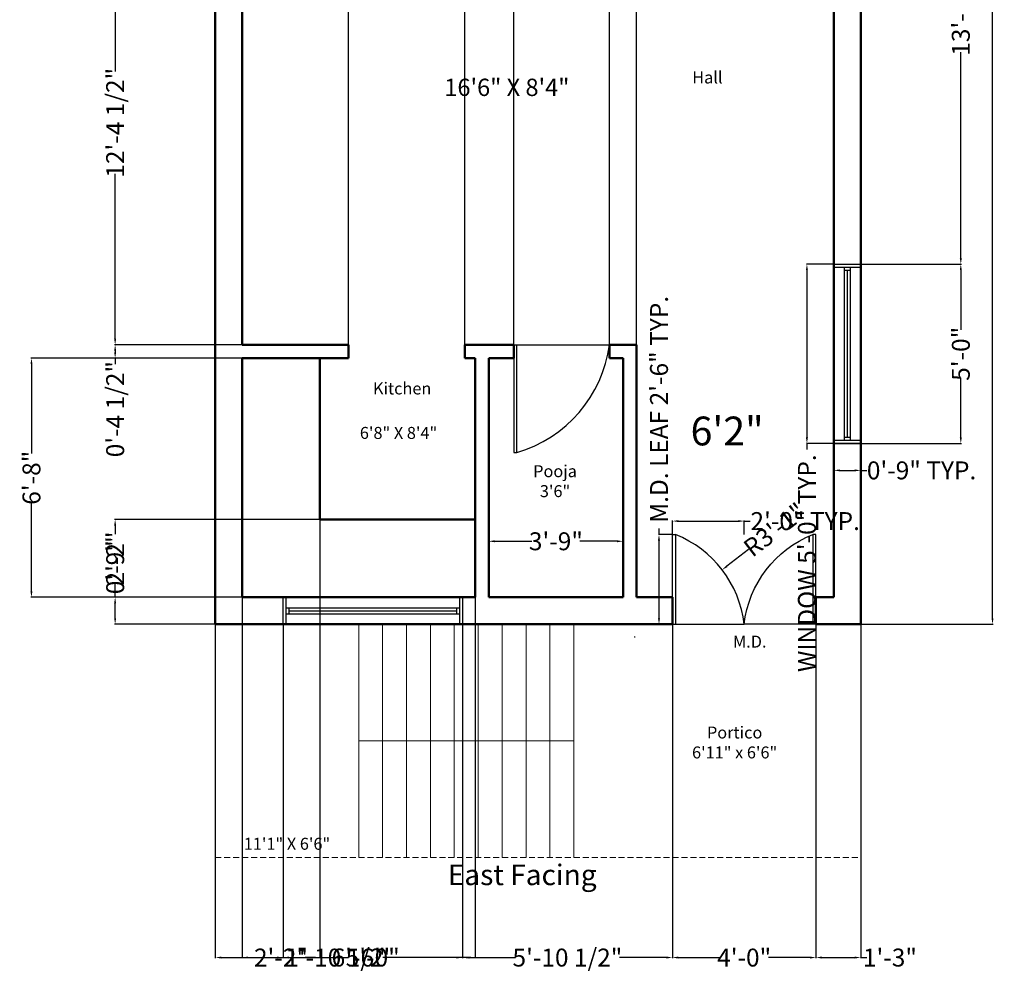
# Model space of a CAD drawing. Units: inches. Extents: x -34 to 296, y -84 to 618.
# Tile 1 of 3: x -34 to 296, y -84 to 238. Entities that reach past the tile are written whole.
import ezdxf

# ---------------------------------------------------------------- set-up
doc = ezdxf.new("R2010")
doc.units = ezdxf.units.IN
doc.header["$LTSCALE"] = 4
doc.header["$MEASUREMENT"] = 0
doc.linetypes.add('DASHED', pattern=[0.75, 0.5, -0.25])
for name, color, linetype, lineweight in [('A-ANNO-DIMS', 2, 'Continuous', 18), ('A-ANNO-TEXT', 7, 'Continuous', 18), ('A-AREA-IDEN', 3, 'Continuous', 18), ('A-DOOR', 4, 'Continuous', 25), ('A-FLOR-OVHD', 8, 'DASHED', 18), ('A-FLOR-STRS', 8, 'Continuous', 18), ('A-GLAZ', 3, 'Continuous', 25), ('A-WALL', 7, 'Continuous', 50)]:
    doc.layers.add(name, color=color, linetype=linetype, lineweight=lineweight)
doc.styles.get("Standard").update_dxf_attribs({"font": 'arial.ttf'})
doc.dimstyles.get("Standard").update_dxf_attribs({"dimtxt": 6, "dimasz": 2, "dimexe": 0.18, "dimexo": 0.0625, "dimgap": 0.09, "dimtad": 0, "dimdec": 0, "dimzin": 0, "dimdsep": 46, "dimlunit": 4, "dimtxsty": 'Standard', "dimcen": 0.09, "dimadec": 0, "dimazin": 0, "dimtfac": 1, "dimtdec": 0, "dimtofl": 0, "dimtmove": 0, "dimatfit": 3, "dimfxl": 1, "dimtolj": 1, "dimtzin": 0, "dimarcsym": 0})

# ---------------------------------------------------------------- blocks, each defined once
blk = doc.blocks.new('*D2')
at = {"layer": 'A-ANNO-DIMS', "color": 0, "lineweight": -2, "transparency": 16777216}
for p, q in [((247.53, 576.03), (291.77, 576.03)), ((291.59, 574.03), (291.59, 311.33)), ((291.59, 38.03), (291.59, 300.73)), ((247.53, 36.03), (291.77, 36.03))]:
    blk.add_line(p, q, dxfattribs=at)
at = {"layer": 'A-ANNO-DIMS', "color": 0, "transparency": 16777216}
for points in [[(291.26, 574.03), (291.92, 574.03), (291.59, 576.03)], [(291.26, 38.03), (291.92, 38.03), (291.59, 36.03)]]:
    blk.add_solid(points, dxfattribs=at)
at = {"layer": 'Defpoints', "color": 0, "transparency": 16777216}
for p in [(247.47, 576.03), (247.47, 36.03), (291.59, 36.03)]:
    blk.add_point(p, dxfattribs=at)
at = {"layer": 'A-ANNO-DIMS', "color": 0, "transparency": 16777216, "insert": (291.59, 306.03), "char_height": 6, "attachment_point": 5, "rotation": 90}
blk.add_mtext("\\A1;45'", dxfattribs=at)
blk = doc.blocks.new('*D3')
at = {"layer": 'A-ANNO-DIMS', "color": 0, "lineweight": -2, "transparency": 16777216}
for p, q in [((40.4, 125.03), (-30.22, 125.03)), ((-30.04, 123.03), (-30.04, 93.11)), ((-30.04, 47.03), (-30.04, 76.95)), ((40.4, 45.03), (-30.22, 45.03))]:
    blk.add_line(p, q, dxfattribs=at)
at = {"layer": 'A-ANNO-DIMS', "color": 0, "transparency": 16777216}
for points in [[(-30.37, 123.03), (-29.7, 123.03), (-30.04, 125.03)], [(-30.37, 47.03), (-29.7, 47.03), (-30.04, 45.03)]]:
    blk.add_solid(points, dxfattribs=at)
at = {"layer": 'Defpoints', "color": 0, "transparency": 16777216}
for p in [(-30.04, 125.03), (40.47, 125.03), (40.47, 45.03)]:
    blk.add_point(p, dxfattribs=at)
at = {"layer": 'A-ANNO-DIMS', "color": 0, "transparency": 16777216, "insert": (-30.04, 85.03), "char_height": 6, "attachment_point": 5, "rotation": 90}
blk.add_mtext('\\A1;6\'-8"', dxfattribs=at)
blk = doc.blocks.new('*D4')
at = {"layer": 'A-ANNO-DIMS', "color": 0, "lineweight": -2, "transparency": 16777216}
for p, q in [((122.97, 45.1), (122.97, 63.96)), ((124.97, 63.78), (137.4, 63.78)), ((165.97, 63.78), (153.53, 63.78)), ((167.97, 45.1), (167.97, 63.96))]:
    blk.add_line(p, q, dxfattribs=at)
at = {"layer": 'A-ANNO-DIMS', "color": 0, "transparency": 16777216}
for points in [[(124.97, 64.11), (124.97, 63.45), (122.97, 63.78)], [(165.97, 64.11), (165.97, 63.45), (167.97, 63.78)]]:
    blk.add_solid(points, dxfattribs=at)
at = {"layer": 'Defpoints', "color": 0, "transparency": 16777216}
for p in [(122.97, 63.78), (122.97, 45.03), (167.97, 45.03)]:
    blk.add_point(p, dxfattribs=at)
at = {"layer": 'A-ANNO-DIMS', "color": 0, "transparency": 16777216, "insert": (145.47, 63.78), "char_height": 6, "attachment_point": 5}
blk.add_mtext('\\A1;3\'-9"', dxfattribs=at)
blk = doc.blocks.new('DOOR')
for p, q in [((177.71, 683.29), (177.71, 692.29)), ((177.71, 692.29), (237.71, 692.29)), ((178.71, 683.29), (178.71, 692.29)), ((236.71, 692.29), (236.71, 683.29)), ((237.71, 692.29), (237.71, 683.29)), ((178.71, 688.79), (236.71, 688.79)), ((179.71, 686.79), (179.71, 688.79)), ((235.71, 688.79), (235.71, 686.79)), ((178.71, 686.79), (236.71, 686.79)), ((179.71, 687.79), (235.71, 687.79)), ((237.71, 683.29), (177.71, 683.29))]:
    blk.add_line(p, q)
blk = doc.blocks.new('DOOR-600-LEAF')
for p, q in [((0, 0), (0, 30)), ((0, 30), (1, 30)), ((1, 30), (1, 0)), ((0, 0), (24, 0))]:
    blk.add_line(p, q)
blk.add_arc((-12.59, -4.23), 36.83, 6.598, 68.3543)
blk = doc.blocks.new('*D8')
at = {"layer": 'A-ANNO-DIMS', "color": 0, "lineweight": -2, "transparency": 16777216}
for p, q in [((238.4, 156.5), (229.29, 156.5)), ((229.47, 154.5), (229.47, 98.5)), ((238.4, 96.5), (229.29, 96.5)), ((229.47, 96.5), (229.47, 94.5))]:
    blk.add_line(p, q, dxfattribs=at)
at = {"layer": 'A-ANNO-DIMS', "color": 0, "transparency": 16777216}
for points in [[(229.13, 154.5), (229.8, 154.5), (229.47, 156.5)], [(229.13, 98.5), (229.8, 98.5), (229.47, 96.5)]]:
    blk.add_solid(points, dxfattribs=at)
at = {"layer": 'Defpoints', "color": 0, "transparency": 16777216}
for p in [(238.47, 156.5), (229.47, 96.5), (238.47, 96.5)]:
    blk.add_point(p, dxfattribs=at)
at = {"layer": 'A-ANNO-DIMS', "color": 0, "transparency": 16777216, "insert": (229.47, 56.44), "char_height": 6, "attachment_point": 5, "rotation": 90}
blk.add_mtext('\\A1;WINDOW 5\'-0" TYP.', dxfattribs=at)
blk = doc.blocks.new('*D9')
at = {"layer": 'A-ANNO-DIMS', "color": 0, "lineweight": -2, "transparency": 16777216}
for p, q in [((238.47, 96.43), (238.47, 87.32)), ((247.47, 96.43), (247.47, 87.32)), ((240.47, 87.5), (245.47, 87.5)), ((247.47, 87.5), (249.47, 87.5))]:
    blk.add_line(p, q, dxfattribs=at)
at = {"layer": 'A-ANNO-DIMS', "color": 0, "transparency": 16777216}
for points in [[(240.47, 87.83), (240.47, 87.16), (238.47, 87.5)], [(245.47, 87.83), (245.47, 87.16), (247.47, 87.5)]]:
    blk.add_solid(points, dxfattribs=at)
at = {"layer": 'Defpoints', "color": 0, "transparency": 16777216}
for p in [(238.47, 96.5), (247.47, 96.5), (247.47, 87.5)]:
    blk.add_point(p, dxfattribs=at)
at = {"layer": 'A-ANNO-DIMS', "color": 0, "transparency": 16777216, "insert": (267.84, 87.5), "char_height": 6, "attachment_point": 5}
blk.add_mtext('\\A1;0\'-9" TYP.', dxfattribs=at)
blk = doc.blocks.new('*D12')
at = {"layer": 'A-ANNO-DIMS', "color": 0, "lineweight": -2, "transparency": 16777216}
for p, q in [((184.4, 66.03), (179.79, 66.03)), ((179.97, 66.03), (179.97, 68.03)), ((179.97, 38.03), (179.97, 64.03)), ((184.4, 36.03), (179.79, 36.03))]:
    blk.add_line(p, q, dxfattribs=at)
at = {"layer": 'A-ANNO-DIMS', "color": 0, "transparency": 16777216}
for points in [[(179.63, 64.03), (180.3, 64.03), (179.97, 66.03)], [(179.63, 38.03), (180.3, 38.03), (179.97, 36.03)]]:
    blk.add_solid(points, dxfattribs=at)
at = {"layer": 'Defpoints', "color": 0, "transparency": 16777216}
for p in [(179.97, 66.03), (184.47, 66.03), (184.47, 36.03)]:
    blk.add_point(p, dxfattribs=at)
at = {"layer": 'A-ANNO-DIMS', "color": 0, "transparency": 16777216, "insert": (179.97, 107.93), "char_height": 6, "attachment_point": 5, "rotation": 90}
blk.add_mtext('\\A1;M.D. LEAF 2\'-6" TYP.', dxfattribs=at)
blk = doc.blocks.new('*D13')
at = {"layer": 'A-ANNO-DIMS', "color": 0, "lineweight": -2, "transparency": 16777216}
for p, q in [((184.47, 66.1), (184.47, 70.71)), ((186.47, 70.53), (206.47, 70.53)), ((208.47, 66.1), (208.47, 70.71)), ((208.47, 70.53), (210.47, 70.53))]:
    blk.add_line(p, q, dxfattribs=at)
at = {"layer": 'A-ANNO-DIMS', "color": 0, "transparency": 16777216}
for points in [[(186.47, 70.87), (186.47, 70.2), (184.47, 70.53)], [(206.47, 70.87), (206.47, 70.2), (208.47, 70.53)]]:
    blk.add_solid(points, dxfattribs=at)
at = {"layer": 'Defpoints', "color": 0, "transparency": 16777216}
for p in [(208.47, 70.53), (184.47, 66.03), (208.47, 66.03)]:
    blk.add_point(p, dxfattribs=at)
at = {"layer": 'A-ANNO-DIMS', "color": 0, "transparency": 16777216, "insert": (228.89, 70.53), "char_height": 6, "attachment_point": 5}
blk.add_mtext('\\A1;2\'-0" TYP.', dxfattribs=at)
blk = doc.blocks.new('*D28')
at = {"layer": 'A-ANNO-DIMS', "color": 0, "lineweight": -2, "transparency": 16777216}
for p, q in [((40.4, 278.03), (-2.21, 278.03)), ((-2.03, 276.03), (-2.03, 220.89)), ((-2.03, 131.53), (-2.03, 186.68)), ((40.4, 129.53), (-2.21, 129.53))]:
    blk.add_line(p, q, dxfattribs=at)
at = {"layer": 'A-ANNO-DIMS', "color": 0, "transparency": 16777216}
for points in [[(-2.37, 276.03), (-1.7, 276.03), (-2.03, 278.03)], [(-2.37, 131.53), (-1.7, 131.53), (-2.03, 129.53)]]:
    blk.add_solid(points, dxfattribs=at)
at = {"layer": 'Defpoints', "color": 0, "transparency": 16777216}
for p in [(40.47, 278.03), (-2.03, 129.53), (40.47, 129.53)]:
    blk.add_point(p, dxfattribs=at)
at = {"layer": 'A-ANNO-DIMS', "color": 0, "transparency": 16777216, "insert": (-2.03, 203.78), "char_height": 6, "attachment_point": 5, "rotation": 90}
blk.add_mtext('\\A1;12\'-4 1/2"', dxfattribs=at)
blk = doc.blocks.new('*D39')
at = {"layer": 'A-ANNO-DIMS', "color": 0, "lineweight": -2, "transparency": 16777216}
for p, q in [((164.53, 318.53), (281.15, 318.53)), ((280.97, 316.53), (280.97, 247.63)), ((280.97, 158.5), (280.97, 227.4)), ((238.53, 156.5), (281.15, 156.5))]:
    blk.add_line(p, q, dxfattribs=at)
at = {"layer": 'A-ANNO-DIMS', "color": 0, "transparency": 16777216}
for points in [[(280.63, 316.53), (281.3, 316.53), (280.97, 318.53)], [(280.63, 158.5), (281.3, 158.5), (280.97, 156.5)]]:
    blk.add_solid(points, dxfattribs=at)
at = {"layer": 'Defpoints', "color": 0, "transparency": 16777216}
for p in [(164.47, 318.53), (238.47, 156.5), (280.97, 156.5)]:
    blk.add_point(p, dxfattribs=at)
at = {"layer": 'A-ANNO-DIMS', "color": 0, "transparency": 16777216, "insert": (280.97, 237.51), "char_height": 6, "attachment_point": 5, "rotation": 90}
blk.add_mtext('\\A1;13\'-6"', dxfattribs=at)
blk = doc.blocks.new('*D40')
at = {"layer": 'A-ANNO-DIMS', "color": 0, "lineweight": -2, "transparency": 16777216}
for p, q in [((238.53, 156.5), (281.15, 156.5)), ((280.97, 154.5), (280.97, 134.56)), ((280.97, 98.5), (280.97, 118.43)), ((238.53, 96.5), (281.15, 96.5))]:
    blk.add_line(p, q, dxfattribs=at)
at = {"layer": 'A-ANNO-DIMS', "color": 0, "transparency": 16777216}
for points in [[(280.63, 154.5), (281.3, 154.5), (280.97, 156.5)], [(280.63, 98.5), (281.3, 98.5), (280.97, 96.5)]]:
    blk.add_solid(points, dxfattribs=at)
at = {"layer": 'Defpoints', "color": 0, "transparency": 16777216}
for p in [(238.47, 156.5), (238.47, 96.5), (280.97, 96.5)]:
    blk.add_point(p, dxfattribs=at)
at = {"layer": 'A-ANNO-DIMS', "color": 0, "transparency": 16777216, "insert": (280.97, 126.5), "char_height": 6, "attachment_point": 5, "rotation": 90}
blk.add_mtext('\\A1;5\'-0"', dxfattribs=at)
blk = doc.blocks.new('*D44')
at = {"layer": 'A-ANNO-DIMS', "color": 0, "lineweight": -2, "transparency": 16777216}
for p, q in [((31.47, 35.97), (31.47, -75.65)), ((54.17, 35.97), (54.17, -75.65)), ((33.47, -75.47), (52.17, -75.47)), ((54.17, -75.47), (56.17, -75.47))]:
    blk.add_line(p, q, dxfattribs=at)
at = {"layer": 'A-ANNO-DIMS', "color": 0, "transparency": 16777216}
for points in [[(33.47, -75.13), (33.47, -75.8), (31.47, -75.47)], [(52.17, -75.13), (52.17, -75.8), (54.17, -75.47)]]:
    blk.add_solid(points, dxfattribs=at)
at = {"layer": 'Defpoints', "color": 0, "transparency": 16777216}
for p in [(31.47, 36.03), (54.17, 36.03), (54.17, -75.47)]:
    blk.add_point(p, dxfattribs=at)
at = {"layer": 'A-ANNO-DIMS', "color": 0, "transparency": 16777216, "insert": (73.27, -75.47), "char_height": 6, "attachment_point": 5}
blk.add_mtext('\\A1;1\'-10 1/2"', dxfattribs=at)
blk = doc.blocks.new('*D45')
at = {"layer": 'A-ANNO-DIMS', "color": 0, "lineweight": -2, "transparency": 16777216}
for p, q in [((54.17, 35.97), (54.17, -75.65)), ((114.17, 35.97), (114.17, -75.65)), ((56.17, -75.47), (76.1, -75.47)), ((112.17, -75.47), (92.23, -75.47))]:
    blk.add_line(p, q, dxfattribs=at)
at = {"layer": 'A-ANNO-DIMS', "color": 0, "transparency": 16777216}
for points in [[(56.17, -75.13), (56.17, -75.8), (54.17, -75.47)], [(112.17, -75.13), (112.17, -75.8), (114.17, -75.47)]]:
    blk.add_solid(points, dxfattribs=at)
at = {"layer": 'Defpoints', "color": 0, "transparency": 16777216}
for p in [(54.17, 36.03), (114.17, 36.03), (114.17, -75.47)]:
    blk.add_point(p, dxfattribs=at)
at = {"layer": 'A-ANNO-DIMS', "color": 0, "transparency": 16777216, "insert": (84.17, -75.47), "char_height": 6, "attachment_point": 5}
blk.add_mtext('\\A1;5\'-0"', dxfattribs=at)
blk = doc.blocks.new('*D46')
at = {"layer": 'A-ANNO-DIMS', "color": 0, "lineweight": -2, "transparency": 16777216}
for p, q in [((114.17, 35.97), (114.17, -75.65)), ((184.47, 35.97), (184.47, -75.65)), ((116.17, -75.47), (131.93, -75.47)), ((182.47, -75.47), (166.7, -75.47))]:
    blk.add_line(p, q, dxfattribs=at)
at = {"layer": 'A-ANNO-DIMS', "color": 0, "transparency": 16777216}
for points in [[(116.17, -75.13), (116.17, -75.8), (114.17, -75.47)], [(182.47, -75.13), (182.47, -75.8), (184.47, -75.47)]]:
    blk.add_solid(points, dxfattribs=at)
at = {"layer": 'Defpoints', "color": 0, "transparency": 16777216}
for p in [(114.17, 36.03), (184.47, 36.03), (184.47, -75.47)]:
    blk.add_point(p, dxfattribs=at)
at = {"layer": 'A-ANNO-DIMS', "color": 0, "transparency": 16777216, "insert": (149.32, -75.47), "char_height": 6, "attachment_point": 5}
blk.add_mtext('\\A1;5\'-10 1/2"', dxfattribs=at)
blk = doc.blocks.new('*D47')
at = {"layer": 'A-ANNO-DIMS', "color": 0, "lineweight": -2, "transparency": 16777216}
for p, q in [((184.47, 35.97), (184.47, -75.65)), ((232.47, 35.97), (232.47, -75.65)), ((186.47, -75.47), (200.28, -75.47)), ((230.47, -75.47), (216.65, -75.47))]:
    blk.add_line(p, q, dxfattribs=at)
at = {"layer": 'A-ANNO-DIMS', "color": 0, "transparency": 16777216}
for points in [[(186.47, -75.13), (186.47, -75.8), (184.47, -75.47)], [(230.47, -75.13), (230.47, -75.8), (232.47, -75.47)]]:
    blk.add_solid(points, dxfattribs=at)
at = {"layer": 'Defpoints', "color": 0, "transparency": 16777216}
for p in [(184.47, 36.03), (232.47, 36.03), (232.47, -75.47)]:
    blk.add_point(p, dxfattribs=at)
at = {"layer": 'A-ANNO-DIMS', "color": 0, "transparency": 16777216, "insert": (208.47, -75.47), "char_height": 6, "attachment_point": 5}
blk.add_mtext('\\A1;4\'-0"', dxfattribs=at)
blk = doc.blocks.new('*D48')
at = {"layer": 'A-ANNO-DIMS', "color": 0, "lineweight": -2, "transparency": 16777216}
for p, q in [((232.47, 35.97), (232.47, -75.65)), ((247.47, 35.97), (247.47, -75.65)), ((234.47, -75.47), (245.47, -75.47)), ((247.47, -75.47), (249.47, -75.47))]:
    blk.add_line(p, q, dxfattribs=at)
at = {"layer": 'A-ANNO-DIMS', "color": 0, "transparency": 16777216}
for points in [[(234.47, -75.13), (234.47, -75.8), (232.47, -75.47)], [(245.47, -75.13), (245.47, -75.8), (247.47, -75.47)]]:
    blk.add_solid(points, dxfattribs=at)
at = {"layer": 'Defpoints', "color": 0, "transparency": 16777216}
for p in [(232.47, 36.03), (247.47, 36.03), (247.47, -75.47)]:
    blk.add_point(p, dxfattribs=at)
at = {"layer": 'A-ANNO-DIMS', "color": 0, "transparency": 16777216, "insert": (257.25, -75.47), "char_height": 6, "attachment_point": 5}
blk.add_mtext('\\A1;1\'-3"', dxfattribs=at)
blk = doc.blocks.new('*D49')
at = {"layer": 'A-ANNO-DIMS', "color": 0, "lineweight": -2, "transparency": 16777216}
for p, q in [((-2.03, 45.03), (-2.03, 47.03)), ((40.4, 45.03), (-2.21, 45.03)), ((-2.03, 38.03), (-2.03, 43.03)), ((31.4, 36.03), (-2.21, 36.03))]:
    blk.add_line(p, q, dxfattribs=at)
at = {"layer": 'A-ANNO-DIMS', "color": 0, "transparency": 16777216}
for points in [[(-2.37, 43.03), (-1.7, 43.03), (-2.03, 45.03)], [(-2.37, 38.03), (-1.7, 38.03), (-2.03, 36.03)]]:
    blk.add_solid(points, dxfattribs=at)
at = {"layer": 'Defpoints', "color": 0, "transparency": 16777216}
for p in [(-2.03, 45.03), (40.47, 45.03), (31.47, 36.03)]:
    blk.add_point(p, dxfattribs=at)
at = {"layer": 'A-ANNO-DIMS', "color": 0, "transparency": 16777216, "insert": (-2.03, 55.1), "char_height": 6, "attachment_point": 5, "rotation": 90}
blk.add_mtext('\\A1;0\'-9"', dxfattribs=at)
blk = doc.blocks.new('*D50')
at = {"layer": 'A-ANNO-DIMS', "color": 0, "lineweight": -2, "transparency": 16777216}
for p, q in [((40.4, 129.53), (-2.21, 129.53)), ((-2.03, 127.53), (-2.03, 127.03)), ((40.4, 125.03), (-2.21, 125.03)), ((-2.03, 125.03), (-2.03, 123.03))]:
    blk.add_line(p, q, dxfattribs=at)
at = {"layer": 'A-ANNO-DIMS', "color": 0, "transparency": 16777216}
for points in [[(-2.37, 127.53), (-1.7, 127.53), (-2.03, 129.53)], [(-2.37, 127.03), (-1.7, 127.03), (-2.03, 125.03)]]:
    blk.add_solid(points, dxfattribs=at)
at = {"layer": 'Defpoints', "color": 0, "transparency": 16777216}
for p in [(40.47, 129.53), (-2.03, 125.03), (40.47, 125.03)]:
    blk.add_point(p, dxfattribs=at)
at = {"layer": 'A-ANNO-DIMS', "color": 0, "transparency": 16777216, "insert": (-2.03, 107.98), "char_height": 6, "attachment_point": 5, "rotation": 90}
blk.add_mtext('\\A1;0\'-4 1/2"', dxfattribs=at)
blk = doc.blocks.new('*D51')
at = {"layer": 'A-ANNO-DIMS', "color": 0, "lineweight": -2, "transparency": 16777216}
for p, q in [((40.47, 129.6), (40.47, 609.71)), ((76.01, 129.6), (76.01, 609.71)), ((38.47, 609.53), (36.47, 609.53)), ((78.01, 609.53), (80.01, 609.53))]:
    blk.add_line(p, q, dxfattribs=at)
at = {"layer": 'A-ANNO-DIMS', "color": 0, "transparency": 16777216}
for points in [[(38.47, 609.87), (38.47, 609.2), (40.47, 609.53)], [(78.01, 609.87), (78.01, 609.2), (76.01, 609.53)]]:
    blk.add_solid(points, dxfattribs=at)
at = {"layer": 'Defpoints', "color": 0, "transparency": 16777216}
for p in [(76.01, 609.53), (40.47, 129.53), (76.01, 129.53)]:
    blk.add_point(p, dxfattribs=at)
at = {"layer": 'A-ANNO-DIMS', "color": 0, "transparency": 16777216, "insert": (58.24, 609.53), "char_height": 6, "attachment_point": 5}
blk.add_mtext('\\A1;2\'-11 1/2"', dxfattribs=at)
blk = doc.blocks.new('*D52')
at = {"layer": 'A-ANNO-DIMS', "color": 0, "lineweight": -2, "transparency": 16777216}
for p, q in [((76.01, 129.6), (76.01, 609.71)), ((115.01, 129.6), (115.01, 609.71)), ((78.01, 609.53), (87.45, 609.53)), ((113.01, 609.53), (103.57, 609.53))]:
    blk.add_line(p, q, dxfattribs=at)
at = {"layer": 'A-ANNO-DIMS', "color": 0, "transparency": 16777216}
for points in [[(78.01, 609.87), (78.01, 609.2), (76.01, 609.53)], [(113.01, 609.87), (113.01, 609.2), (115.01, 609.53)]]:
    blk.add_solid(points, dxfattribs=at)
at = {"layer": 'Defpoints', "color": 0, "transparency": 16777216}
for p in [(115.01, 609.53), (76.01, 129.53), (115.01, 129.53)]:
    blk.add_point(p, dxfattribs=at)
at = {"layer": 'A-ANNO-DIMS', "color": 0, "transparency": 16777216, "insert": (95.51, 609.53), "char_height": 6, "attachment_point": 5}
blk.add_mtext('\\A1;3\'-3"', dxfattribs=at)
blk = doc.blocks.new('*D53')
at = {"layer": 'A-ANNO-DIMS', "color": 0, "lineweight": -2, "transparency": 16777216}
for p, q in [((115.01, 129.6), (115.01, 609.71)), ((131.36, 129.6), (131.36, 609.71)), ((117.01, 609.53), (129.36, 609.53)), ((131.36, 609.53), (133.36, 609.53))]:
    blk.add_line(p, q, dxfattribs=at)
at = {"layer": 'A-ANNO-DIMS', "color": 0, "transparency": 16777216}
for points in [[(117.01, 609.87), (117.01, 609.2), (115.01, 609.53)], [(129.36, 609.87), (129.36, 609.2), (131.36, 609.53)]]:
    blk.add_solid(points, dxfattribs=at)
at = {"layer": 'Defpoints', "color": 0, "transparency": 16777216}
for p in [(131.36, 609.53), (115.01, 129.53), (131.36, 129.53)]:
    blk.add_point(p, dxfattribs=at)
at = {"layer": 'A-ANNO-DIMS', "color": 0, "transparency": 16777216, "insert": (148.13, 609.53), "char_height": 6, "attachment_point": 5}
blk.add_mtext('\\A1;1\'-4 1/2"', dxfattribs=at)
blk = doc.blocks.new('*D54')
at = {"layer": 'A-ANNO-DIMS', "color": 0, "lineweight": -2, "transparency": 16777216}
for p, q in [((131.36, 129.6), (131.36, 609.71)), ((163.36, 129.6), (163.36, 609.71)), ((133.36, 609.53), (139.24, 609.53)), ((161.36, 609.53), (155.48, 609.53))]:
    blk.add_line(p, q, dxfattribs=at)
at = {"layer": 'A-ANNO-DIMS', "color": 0, "transparency": 16777216}
for points in [[(133.36, 609.87), (133.36, 609.2), (131.36, 609.53)], [(161.36, 609.87), (161.36, 609.2), (163.36, 609.53)]]:
    blk.add_solid(points, dxfattribs=at)
at = {"layer": 'Defpoints', "color": 0, "transparency": 16777216}
for p in [(163.36, 609.53), (131.36, 129.53), (163.36, 129.53)]:
    blk.add_point(p, dxfattribs=at)
at = {"layer": 'A-ANNO-DIMS', "color": 0, "transparency": 16777216, "insert": (147.36, 609.53), "char_height": 6, "attachment_point": 5}
blk.add_mtext('\\A1;2\'-8"', dxfattribs=at)
blk = doc.blocks.new('*D55')
at = {"layer": 'A-ANNO-DIMS', "color": 0, "lineweight": -2, "transparency": 16777216}
for p, q in [((163.36, 129.6), (163.36, 609.71)), ((172.47, 129.6), (172.47, 609.71)), ((165.36, 609.53), (170.47, 609.53)), ((172.47, 609.53), (174.47, 609.53))]:
    blk.add_line(p, q, dxfattribs=at)
at = {"layer": 'A-ANNO-DIMS', "color": 0, "transparency": 16777216}
for points in [[(165.36, 609.87), (165.36, 609.2), (163.36, 609.53)], [(170.47, 609.87), (170.47, 609.2), (172.47, 609.53)]]:
    blk.add_solid(points, dxfattribs=at)
at = {"layer": 'Defpoints', "color": 0, "transparency": 16777216}
for p in [(172.47, 609.53), (163.36, 129.53), (172.47, 129.53)]:
    blk.add_point(p, dxfattribs=at)
at = {"layer": 'A-ANNO-DIMS', "color": 0, "transparency": 16777216, "insert": (182.53, 609.53), "char_height": 6, "attachment_point": 5}
blk.add_mtext('\\A1;0\'-9"', dxfattribs=at)
blk = doc.blocks.new('*D56')
at = {"layer": 'A-ANNO-DIMS', "color": 0, "lineweight": -2, "transparency": 16777216}
for p, q in [((40.47, 124.97), (40.47, -75.65)), ((118.47, 124.97), (118.47, -75.65)), ((42.47, -75.47), (71.39, -75.47)), ((116.47, -75.47), (87.55, -75.47))]:
    blk.add_line(p, q, dxfattribs=at)
at = {"layer": 'A-ANNO-DIMS', "color": 0, "transparency": 16777216}
for points in [[(42.47, -75.13), (42.47, -75.8), (40.47, -75.47)], [(116.47, -75.13), (116.47, -75.8), (118.47, -75.47)]]:
    blk.add_solid(points, dxfattribs=at)
at = {"layer": 'Defpoints', "color": 0, "transparency": 16777216}
for p in [(40.47, 125.03), (118.47, 125.03), (118.47, -75.47)]:
    blk.add_point(p, dxfattribs=at)
at = {"layer": 'A-ANNO-DIMS', "color": 0, "transparency": 16777216, "insert": (79.47, -75.47), "char_height": 6, "attachment_point": 5}
blk.add_mtext('\\A1;6\'-6"', dxfattribs=at)
blk = doc.blocks.new('*D57')
at = {"layer": 'A-ANNO-DIMS', "color": 0, "lineweight": -2, "transparency": 16777216}
for p, q in [((118.4, 71.03), (-2.21, 71.03)), ((-2.03, 69.03), (-2.03, 66.15)), ((-2.03, 47.03), (-2.03, 49.92)), ((118.4, 45.03), (-2.21, 45.03))]:
    blk.add_line(p, q, dxfattribs=at)
at = {"layer": 'A-ANNO-DIMS', "color": 0, "transparency": 16777216}
for points in [[(-2.37, 69.03), (-1.7, 69.03), (-2.03, 71.03)], [(-2.37, 47.03), (-1.7, 47.03), (-2.03, 45.03)]]:
    blk.add_solid(points, dxfattribs=at)
at = {"layer": 'Defpoints', "color": 0, "transparency": 16777216}
for p in [(-2.03, 71.03), (118.47, 71.03), (118.47, 45.03)]:
    blk.add_point(p, dxfattribs=at)
at = {"layer": 'A-ANNO-DIMS', "color": 0, "transparency": 16777216, "insert": (-2.03, 58.03), "char_height": 6, "attachment_point": 5, "rotation": 90}
blk.add_mtext('\\A1;2\'-2"', dxfattribs=at)
blk = doc.blocks.new('*D58')
at = {"layer": 'A-ANNO-DIMS', "color": 0, "lineweight": -2, "transparency": 16777216}
for p, q in [((66.47, 70.97), (66.47, -75.65)), ((40.47, 44.97), (40.47, -75.65)), ((42.47, -75.47), (45.35, -75.47)), ((64.47, -75.47), (61.58, -75.47))]:
    blk.add_line(p, q, dxfattribs=at)
at = {"layer": 'A-ANNO-DIMS', "color": 0, "transparency": 16777216}
for points in [[(42.47, -75.13), (42.47, -75.8), (40.47, -75.47)], [(64.47, -75.13), (64.47, -75.8), (66.47, -75.47)]]:
    blk.add_solid(points, dxfattribs=at)
at = {"layer": 'Defpoints', "color": 0, "transparency": 16777216}
for p in [(66.47, 71.03), (40.47, 45.03), (66.47, -75.47)]:
    blk.add_point(p, dxfattribs=at)
at = {"layer": 'A-ANNO-DIMS', "color": 0, "transparency": 16777216, "insert": (53.47, -75.47), "char_height": 6, "attachment_point": 5}
blk.add_mtext('\\A1;2\'-2"', dxfattribs=at)
blk = doc.blocks.new('*D60')
at = {"layer": 'A-ANNO-DIMS', "color": 0, "lineweight": -2, "transparency": 16777216}
for p, q in [((209.97, 61), (202.7, 55.43)), ((171.79, 31.8), (171.97, 31.8)), ((171.88, 31.71), (171.88, 31.89))]:
    blk.add_line(p, q, dxfattribs=at)
at = {"layer": 'A-ANNO-DIMS', "color": 0, "transparency": 16777216}
blk.add_solid([(202.49, 55.69), (202.9, 55.16), (201.11, 54.21)], dxfattribs=at)
at = {"layer": 'Defpoints', "color": 0, "transparency": 16777216}
for p in [(201.11, 54.21), (171.88, 31.8)]:
    blk.add_point(p, dxfattribs=at)
at = {"layer": 'A-ANNO-DIMS', "color": 0, "transparency": 16777216, "insert": (218.65, 67.65), "char_height": 6, "attachment_point": 5, "rotation": 37.477}
blk.add_mtext('\\A1;R3\'-1"', dxfattribs=at)

msp = doc.modelspace()

# ---------------------------------------------------------------- linework, layer by layer
at = {"layer": 'A-DOOR'}
for p, q in [((131.36, 129.53), (131.36, 93.53)), ((131.36, 129.53), (163.36, 129.53)), ((132.36, 93.53), (132.36, 129.53)), ((131.36, 93.53), (132.36, 93.53))]:
    msp.add_line(p, q, dxfattribs=at)
msp.add_arc((120.37, 135.21), 43.37, 286.0562, 352.4796, dxfattribs=at)
at = {"layer": 'A-FLOR-OVHD'}
for p, q in [((31.47, 36.03), (31.47, -41.97)), ((247.47, -41.97), (247.47, 36.03)), ((31.47, -41.97), (247.47, -41.97))]:
    msp.add_line(p, q, dxfattribs=at)
at = {"layer": 'A-FLOR-STRS'}
for p, q in [((79.47, 36.03), (79.47, -41.97)), ((87.47, 36.03), (87.47, -41.97)), ((95.47, 36.03), (95.47, -41.97)), ((103.47, 36.03), (103.47, -41.97)), ((111.47, 36.03), (111.47, -41.97)), ((119.47, 36.03), (119.47, -41.97)), ((127.47, 36.03), (127.47, -41.97)), ((135.47, 36.03), (135.47, -41.97)), ((143.47, 36.03), (143.47, -41.97)), ((151.47, 36.03), (151.47, -41.97)), ((79.47, -2.97), (151.47, -2.97))]:
    msp.add_line(p, q, dxfattribs=at)
at = {"layer": 'A-WALL'}
for p, q in [((31.47, 36.03), (31.47, 576.03)), ((247.47, 576.03), (247.47, 36.03)), ((238.47, 468.03), (238.47, 45.03)), ((40.47, 129.53), (40.47, 278.03)), ((76.01, 129.53), (40.47, 129.53)), ((76.01, 125.03), (76.01, 129.53)), ((115.01, 129.53), (115.01, 125.03)), ((131.36, 129.53), (115.01, 129.53)), ((131.36, 125.03), (131.36, 129.53)), ((172.47, 129.53), (163.36, 129.53)), ((163.36, 129.53), (163.36, 125.03)), ((172.47, 45.03), (172.47, 129.53)), ((40.47, 45.03), (40.47, 125.03)), ((76.01, 125.03), (40.47, 125.03)), ((66.47, 71.03), (66.47, 125.03)), ((118.47, 125.03), (115.01, 125.03)), ((118.47, 45.03), (118.47, 125.03)), ((122.97, 45.03), (122.97, 125.03)), ((131.36, 125.03), (122.97, 125.03)), ((167.97, 125.03), (163.36, 125.03)), ((167.97, 45.03), (167.97, 125.03)), ((118.47, 71.03), (66.47, 71.03)), ((118.47, 45.03), (40.47, 45.03)), ((167.97, 45.03), (122.97, 45.03)), ((184.47, 45.03), (172.47, 45.03)), ((184.47, 36.03), (184.47, 45.03)), ((238.47, 45.03), (232.47, 45.03)), ((232.47, 45.03), (232.47, 36.03)), ((184.47, 36.03), (31.47, 36.03)), ((247.47, 36.03), (232.47, 36.03))]:
    msp.add_line(p, q, dxfattribs=at)

# ---------------------------------------------------------------- block references
at = {"layer": 'A-DOOR'}
msp.add_blockref('DOOR-600-LEAF', (184.47, 36.03), dxfattribs=at)
at = {"layer": 'A-DOOR', "extrusion": (0, 0, -1), "zscale": -1}
msp.add_blockref('DOOR-600-LEAF', (-232.47, 36.03), dxfattribs=at)
at = {"layer": 'A-GLAZ', "rotation": 270}
msp.add_blockref('DOOR', (-444.82, 334.2), dxfattribs=at)
at = {"layer": 'A-GLAZ'}
msp.add_blockref('DOOR', (-123.54, -647.26), dxfattribs=at)

# ---------------------------------------------------------------- texts
at = {"layer": 'A-ANNO-TEXT', "insert": (24.7, -44.35), "char_height": 6.8966, "attachment_point": 1}
msp.add_mtext_dynamic_manual_height_columns('\\pxqc;East Facing', width=218.9903, gutter_width=34.48, heights=[0], dxfattribs=at)
at = {"layer": 'A-AREA-IDEN', "attachment_point": 1}
for s, width, gutter_width, insert, char_height in [('\\pxqc;Hall', 54.181, 20, (169.08, 220.93), 4), ('\\pxqc;16\'6" X 8\'4"', 154.3935, 28.96, (51.86, 218.52), 5.791), ('\\pxqc;Kitchen ', 41.2195, 20, (73.41, 116.9), 4), ('\\pxqc;6\'2"', 104.4689, 48.17, (150.54, 105.49), 9.633), ('\\pxqc;6\'8" X 8\'4"', 42.624, 20, (71.5, 102.03), 4), ('\\pxqc;Pooja \\P3\'6"', 35.6484, 20, (127.36, 89.22), 4), ('\\pxqc;M.D.', 19.7512, 20, (200.46, 32.22), 4), ('\\pxqc;Portico\\P6\'11" x 6\'6"', 55.8484, 20, (177.36, 1.81), 4), ('\\pxqc;11\'1" X 6\'6"', 43.3968, 20, (33.78, -35.41), 4)]:
    msp.add_mtext_dynamic_manual_height_columns(s, width=width, gutter_width=gutter_width, heights=[0], dxfattribs=dict(at, insert=insert, char_height=char_height))

# ---------------------------------------------------------------- dimensions: what is measured, and where the dimension line sits
at = {"layer": 'A-ANNO-DIMS'}
for base, p1, p2, override, picture, middle in [((76.01, 609.53), (40.47, 129.53), (76.01, 129.53), {"dimdec": 1, "dimlfac": 1, "dimrnd": 0, "dimzin": 1, "dimdsep": 46, "dimlunit": 4, "dimfrac": 2}, '*D51', (58.24, 609.53)), ((131.3602, 609.5325), (115.0111, 129.5325), (131.3602, 129.5325), {"dimdec": 1, "dimlfac": 1, "dimrnd": 0, "dimzin": 1, "dimdsep": 46, "dimlunit": 4, "dimfrac": 2}, '*D53', (148.133, 609.5325)), ((115.01, 609.53), (76.01, 129.53), (115.01, 129.53), {"dimdec": 1, "dimlfac": 1, "dimrnd": 0, "dimzin": 1, "dimdsep": 46, "dimlunit": 4, "dimfrac": 2}, '*D52', (95.51, 609.53)), ((163.36, 609.53), (131.36, 129.53), (163.36, 129.53), {"dimdec": 1, "dimlfac": 1, "dimrnd": 0, "dimzin": 1, "dimdsep": 46, "dimlunit": 4, "dimfrac": 2}, '*D54', (147.36, 609.53)), ((172.47, 609.53), (163.36, 129.53), (172.47, 129.53), {"dimdec": 1, "dimlfac": 1, "dimrnd": 0, "dimzin": 1, "dimdsep": 46, "dimlunit": 4, "dimfrac": 2}, '*D55', (182.53, 609.53)), ((118.47, -75.47), (40.47, 125.03), (118.47, 125.03), {"dimdec": 1, "dimlfac": 1, "dimrnd": 0, "dimzin": 1, "dimdsep": 46, "dimlunit": 4, "dimfrac": 2}, '*D56', (79.47, -75.47)), ((66.47, -75.47), (40.47, 45.03), (66.47, 71.03), {"dimdec": 1, "dimlfac": 1, "dimrnd": 0, "dimzin": 1, "dimdsep": 46, "dimlunit": 4, "dimfrac": 2}, '*D58', (53.47, -75.47)), ((122.97, 63.78), (167.97, 45.03), (122.97, 45.03), {"dimclrd": 0, "dimclre": 0, "dimclrt": 0}, '*D4', (145.47, 63.78)), ((54.17, -75.47), (31.47, 36.03), (54.17, 36.03), {"dimdec": 1, "dimlfac": 1, "dimrnd": 0, "dimzin": 1, "dimdsep": 46, "dimlunit": 4, "dimfrac": 2}, '*D44', (73.27, -75.47)), ((114.17, -75.47), (54.17, 36.03), (114.17, 36.03), {"dimdec": 1, "dimlfac": 1, "dimrnd": 0, "dimzin": 1, "dimdsep": 46, "dimlunit": 4, "dimfrac": 2}, '*D45', (84.17, -75.47)), ((184.47, -75.47), (114.17, 36.03), (184.47, 36.03), {"dimdec": 1, "dimlfac": 1, "dimrnd": 0, "dimzin": 1, "dimdsep": 46, "dimlunit": 4, "dimfrac": 2}, '*D46', (149.32, -75.47)), ((232.47, -75.47), (184.47, 36.03), (232.47, 36.03), {"dimdec": 1, "dimlfac": 1, "dimrnd": 0, "dimzin": 1, "dimdsep": 46, "dimlunit": 4, "dimfrac": 2}, '*D47', (208.47, -75.47)), ((247.47, -75.47), (232.47, 36.03), (247.47, 36.03), {"dimdec": 1, "dimlfac": 1, "dimrnd": 0, "dimzin": 1, "dimdsep": 46, "dimlunit": 4, "dimfrac": 2}, '*D48', (257.25, -75.47))]:
    dim = msp.add_linear_dim(base=base, p1=p1, p2=p2, dimstyle='Standard', override=override, dxfattribs=at)
    dim.commit()
    dim.dimension.update_dxf_attribs({"geometry": picture, "text_midpoint": middle})
for base, p1, p2, override, picture, middle in [((291.59, 36.03), (247.47, 576.03), (247.47, 36.03), {"dimclrd": 0, "dimclre": 0, "dimclrt": 0}, '*D2', (291.59, 306.03)), ((280.97, 156.5), (164.47, 318.53), (238.47, 156.5), {"dimdec": 1, "dimlfac": 1, "dimrnd": 0, "dimzin": 1, "dimdsep": 46, "dimlunit": 4, "dimfrac": 2}, '*D39', (280.97, 237.51)), ((-2.03, 129.53), (40.47, 278.03), (40.47, 129.53), {"dimdec": 1, "dimlfac": 1, "dimrnd": 0, "dimzin": 1, "dimdsep": 46, "dimlunit": 4, "dimfrac": 2}, '*D28', (-2.03, 203.78)), ((280.97, 96.5), (238.47, 156.5), (238.47, 96.5), {"dimdec": 1, "dimlfac": 1, "dimrnd": 0, "dimzin": 1, "dimdsep": 46, "dimlunit": 4, "dimfrac": 2}, '*D40', (280.97, 126.5)), ((-2.03, 125.03), (40.47, 129.53), (40.47, 125.03), {"dimdec": 1, "dimlfac": 1, "dimrnd": 0, "dimzin": 1, "dimdsep": 46, "dimlunit": 4, "dimfrac": 2}, '*D50', (-2.03, 107.98)), ((-30.04, 125.03), (40.47, 45.03), (40.47, 125.03), {"dimclrd": 0, "dimclre": 0, "dimclrt": 0}, '*D3', (-30.04, 85.03)), ((-2.03, 71.03), (118.47, 45.03), (118.47, 71.03), {"dimdec": 1, "dimlfac": 1, "dimrnd": 0, "dimzin": 1, "dimdsep": 46, "dimlunit": 4, "dimfrac": 2}, '*D57', (-2.03, 58.03)), ((-2.03, 45.03), (31.47, 36.03), (40.47, 45.03), {"dimdec": 1, "dimlfac": 1, "dimrnd": 0, "dimzin": 1, "dimdsep": 46, "dimlunit": 4, "dimfrac": 2}, '*D49', (-2.03, 55.1))]:
    dim = msp.add_linear_dim(base=base, p1=p1, p2=p2, angle=90, dimstyle='Standard', override=override, dxfattribs=at)
    dim.commit()
    dim.dimension.update_dxf_attribs({"geometry": picture, "text_midpoint": middle})
for base, p1, p2, angle, text, picture, middle in [((229.47, 96.5), (238.47, 156.5), (238.47, 96.5), 270, 'WINDOW <> TYP.', '*D8', (229.47, 56.44)), ((179.97, 66.03), (184.47, 36.03), (184.47, 66.03), 90, 'M.D. LEAF <> TYP.', '*D12', (179.97, 107.93))]:
    dim = msp.add_linear_dim(base=base, p1=p1, p2=p2, angle=angle, text=text, dimstyle='Standard', override={"dimdec": 1, "dimrnd": 0, "dimzin": 1, "dimlunit": 4, "dimfrac": 2}, dxfattribs=at)
    dim.commit()
    dim.dimension.update_dxf_attribs({"geometry": picture, "text_midpoint": middle})
for base, p1, p2, picture, middle in [((247.47, 87.5), (238.47, 96.5), (247.47, 96.5), '*D9', (267.84, 87.5)), ((208.47, 70.53), (184.47, 66.03), (208.47, 66.03), '*D13', (228.89, 70.53))]:
    dim = msp.add_linear_dim(base=base, p1=p1, p2=p2, text='<> TYP.', dimstyle='Standard', override={"dimdec": 1, "dimrnd": 0, "dimzin": 1, "dimlunit": 4, "dimfrac": 2}, dxfattribs=at)
    dim.commit()
    dim.dimension.update_dxf_attribs({"geometry": picture, "text_midpoint": middle})
dim = msp.add_radius_dim(center=(171.88, 31.8), mpoint=(201.11, 54.21), dimstyle='Standard', override={"dimdec": 1, "dimlfac": 1, "dimrnd": 0, "dimzin": 1, "dimdsep": 46, "dimlunit": 4, "dimfrac": 2}, dxfattribs=at)
dim.commit()
dim.dimension.update_dxf_attribs({"geometry": '*D60', "text_midpoint": (218.65, 67.65), "dimtype": 164})

doc.saveas('drawing.dxf')
